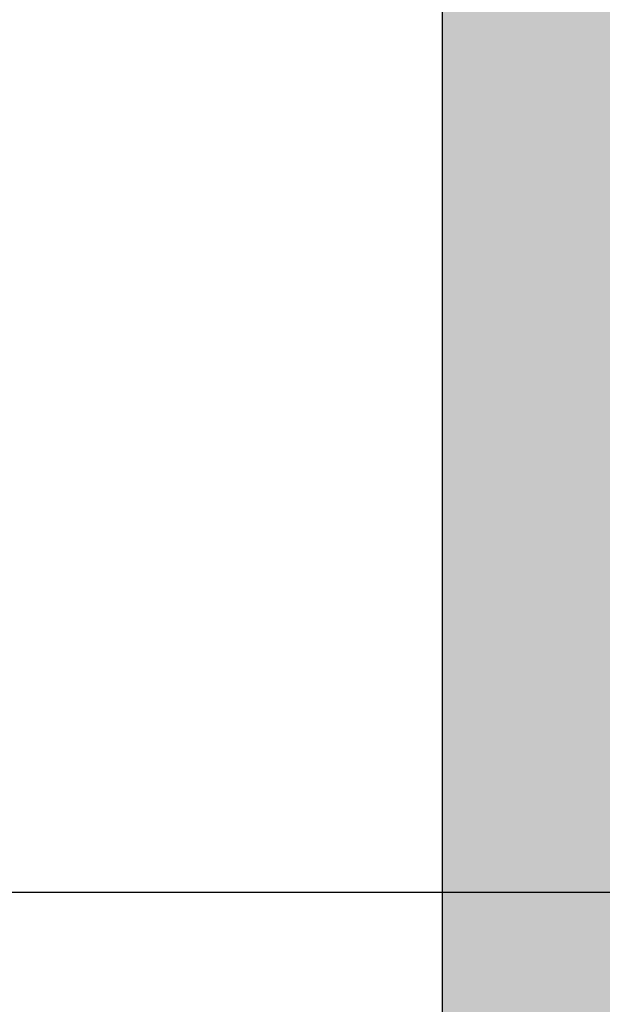
# Model space of a CAD drawing. Units: millimetres. Extents: x -22994 to 29398, y -19990 to 20176.
# Tile 37 of 135: x 190.48 to 197.67, y 29.61 to 41.76. Entities that reach past the tile are written whole.
import ezdxf
from ezdxf import colors
from ezdxf.entities.mleader import LeaderData, LeaderLine
from ezdxf.math import Vec2, Vec3

# ---------------------------------------------------------------- set-up
doc = ezdxf.new("R2010")
doc.units = ezdxf.units.MM
doc.header["$MEASUREMENT"] = 0
for name, color, linetype, lineweight in [('M-ANNO-TEXT', 7, 'Continuous', 25), ('M-DIMS', 2, 'Continuous', 18), ('M-EQPM', 7, 'Continuous', 25), ('M-EQPM-PATT', 7, 'Continuous', 18)]:
    doc.layers.add(name, color=color, linetype=linetype, lineweight=lineweight)
doc.styles.get("Standard").update_dxf_attribs({"font": 'arial.ttf'})
doc.dimstyles.get("Standard").update_dxf_attribs({"dimtxt": 0.18, "dimasz": 10000, "dimexe": 0.18, "dimexo": 0.0625, "dimgap": 0.09, "dimtad": 0, "dimtih": 1, "dimtoh": 1, "dimdec": 0, "dimzin": 0, "dimdsep": 46, "dimtxsty": 'Standard', "dimcen": 0.09, "dimadec": 0, "dimazin": 0, "dimtfac": 1, "dimtdec": 0, "dimtofl": 0, "dimtmove": 0, "dimatfit": 3, "dimfxl": 1, "dimtolj": 1, "dimtzin": 0, "dimlwd": 30, "dimarcsym": 0})

# ---------------------------------------------------------------- blocks, each defined once
blk = doc.blocks.new('*D2')
at = {"layer": 'Defpoints', "color": 0, "transparency": 16777216}
for p in [(6.677, 10.271), (290.852, 10.271), (290.852, -5.079)]:
    blk.add_point(p, dxfattribs=at)
at = {"layer": 'M-DIMS', "color": 0, "lineweight": -2, "transparency": 16777216}
for p, q in [((6.677, 10.209), (6.677, -5.259)), ((290.852, 10.209), (290.852, -5.259))]:
    blk.add_line(p, q, dxfattribs=at)
at = {"layer": 'M-DIMS', "color": 0, "lineweight": 30, "transparency": 16777216}
for p, q in [((-9993.323, -5.079), (-19993.323, -5.079)), ((10290.852, -5.079), (20290.852, -5.079))]:
    blk.add_line(p, q, dxfattribs=at)
at = {"layer": 'M-DIMS', "color": 0, "transparency": 16777216}
for points in [[(-9993.323, 1661.588), (-9993.323, -1671.745), (6.677, -5.079)], [(10290.852, 1661.588), (10290.852, -1671.745), (290.852, -5.079)]]:
    blk.add_solid(points, dxfattribs=at)
at = {"layer": 'M-DIMS', "color": 0, "transparency": 16777216, "insert": (148.765, -5.079), "char_height": 0.18, "attachment_point": 5}
blk.add_mtext('\\A1;284.2', dxfattribs=at)
blk = doc.blocks.new('*D3')
at = {"layer": 'Defpoints', "color": 0, "transparency": 16777216}
for p in [(110.265, 204.165), (110.265, 176.366), (95.833, 127.967)]:
    blk.add_point(p, dxfattribs=at)
at = {"layer": 'M-DIMS', "color": 0, "lineweight": -2, "transparency": 16777216}
for p, q in [((95.833, 128.03), (95.833, 204.345)), ((110.265, 176.429), (110.265, 204.345))]:
    blk.add_line(p, q, dxfattribs=at)
at = {"layer": 'M-DIMS', "color": 0, "lineweight": 30, "transparency": 16777216}
for p, q in [((-9904.167, 204.165), (-19904.167, 204.165)), ((10110.265, 204.165), (20110.265, 204.165))]:
    blk.add_line(p, q, dxfattribs=at)
at = {"layer": 'M-DIMS', "color": 0, "transparency": 16777216}
for points in [[(-9904.167, 1870.832), (-9904.167, -1462.501), (95.833, 204.165)], [(10110.265, 1870.832), (10110.265, -1462.501), (110.265, 204.165)]]:
    blk.add_solid(points, dxfattribs=at)
at = {"layer": 'M-DIMS', "color": 0, "transparency": 16777216, "insert": (103.049, 204.165), "char_height": 0.18, "attachment_point": 5}
blk.add_mtext('\\A1;14.432', dxfattribs=at)
blk = doc.blocks.new('*D4')
at = {"layer": 'Defpoints', "color": 0, "transparency": 16777216}
for p in [(116.265, 204.165), (110.265, 176.366), (116.265, 176.366)]:
    blk.add_point(p, dxfattribs=at)
at = {"layer": 'M-DIMS', "color": 0, "lineweight": -2, "transparency": 16777216}
for p, q in [((110.265, 176.429), (110.265, 204.345)), ((116.265, 176.429), (116.265, 204.345))]:
    blk.add_line(p, q, dxfattribs=at)
at = {"layer": 'M-DIMS', "color": 0, "lineweight": 30, "transparency": 16777216}
for p, q in [((-9889.735, 204.165), (-19889.735, 204.165)), ((10116.265, 204.165), (20116.265, 204.165))]:
    blk.add_line(p, q, dxfattribs=at)
at = {"layer": 'M-DIMS', "color": 0, "transparency": 16777216}
for points in [[(-9889.735, 1870.832), (-9889.735, -1462.501), (110.265, 204.165)], [(10116.265, 1870.832), (10116.265, -1462.501), (116.265, 204.165)]]:
    blk.add_solid(points, dxfattribs=at)
at = {"layer": 'M-DIMS', "color": 0, "transparency": 16777216, "insert": (113.265, 204.165), "char_height": 0.18, "attachment_point": 5}
blk.add_mtext('\\A1;6', dxfattribs=at)
blk = doc.blocks.new('*D5')
at = {"layer": 'Defpoints', "color": 0, "transparency": 16777216}
for p in [(181.265, 204.165), (116.265, 176.366), (181.265, 176.366)]:
    blk.add_point(p, dxfattribs=at)
at = {"layer": 'M-DIMS', "color": 0, "lineweight": -2, "transparency": 16777216}
for p, q in [((116.265, 176.429), (116.265, 204.345)), ((181.265, 176.429), (181.265, 204.345))]:
    blk.add_line(p, q, dxfattribs=at)
at = {"layer": 'M-DIMS', "color": 0, "lineweight": 30, "transparency": 16777216}
for p, q in [((-9883.735, 204.165), (-19883.735, 204.165)), ((10181.265, 204.165), (20181.265, 204.165))]:
    blk.add_line(p, q, dxfattribs=at)
at = {"layer": 'M-DIMS', "color": 0, "transparency": 16777216}
for points in [[(-9883.735, 1870.832), (-9883.735, -1462.501), (116.265, 204.165)], [(10181.265, 1870.832), (10181.265, -1462.501), (181.265, 204.165)]]:
    blk.add_solid(points, dxfattribs=at)
at = {"layer": 'M-DIMS', "color": 0, "transparency": 16777216, "insert": (148.765, 204.165), "char_height": 0.18, "attachment_point": 5}
blk.add_mtext('\\A1;65', dxfattribs=at)
blk = doc.blocks.new('*D6')
at = {"layer": 'Defpoints', "color": 0, "transparency": 16777216}
for p in [(187.265, 204.165), (181.265, 176.366), (187.265, 176.366)]:
    blk.add_point(p, dxfattribs=at)
at = {"layer": 'M-DIMS', "color": 0, "lineweight": -2, "transparency": 16777216}
for p, q in [((181.265, 176.429), (181.265, 204.345)), ((187.265, 176.429), (187.265, 204.345))]:
    blk.add_line(p, q, dxfattribs=at)
at = {"layer": 'M-DIMS', "color": 0, "lineweight": 30, "transparency": 16777216}
for p, q in [((-9818.735, 204.165), (-19818.735, 204.165)), ((10187.265, 204.165), (20187.265, 204.165))]:
    blk.add_line(p, q, dxfattribs=at)
at = {"layer": 'M-DIMS', "color": 0, "transparency": 16777216}
for points in [[(-9818.735, 1870.832), (-9818.735, -1462.501), (181.265, 204.165)], [(10187.265, 1870.832), (10187.265, -1462.501), (187.265, 204.165)]]:
    blk.add_solid(points, dxfattribs=at)
at = {"layer": 'M-DIMS', "color": 0, "transparency": 16777216, "insert": (184.265, 204.165), "char_height": 0.18, "attachment_point": 5}
blk.add_mtext('\\A1;6', dxfattribs=at)
blk = doc.blocks.new('*D7')
at = {"layer": 'Defpoints', "color": 0, "transparency": 16777216}
for p in [(201.697, 204.165), (187.265, 176.366), (201.697, 127.967)]:
    blk.add_point(p, dxfattribs=at)
at = {"layer": 'M-DIMS', "color": 0, "lineweight": -2, "transparency": 16777216}
for p, q in [((187.265, 176.429), (187.265, 204.345)), ((201.697, 128.03), (201.697, 204.345))]:
    blk.add_line(p, q, dxfattribs=at)
at = {"layer": 'M-DIMS', "color": 0, "lineweight": 30, "transparency": 16777216}
for p, q in [((-9812.735, 204.165), (-19812.735, 204.165)), ((10201.697, 204.165), (20201.697, 204.165))]:
    blk.add_line(p, q, dxfattribs=at)
at = {"layer": 'M-DIMS', "color": 0, "transparency": 16777216}
for points in [[(-9812.735, 1870.832), (-9812.735, -1462.501), (187.265, 204.165)], [(10201.697, 1870.832), (10201.697, -1462.501), (201.697, 204.165)]]:
    blk.add_solid(points, dxfattribs=at)
at = {"layer": 'M-DIMS', "color": 0, "transparency": 16777216, "insert": (194.481, 204.165), "char_height": 0.18, "attachment_point": 5}
blk.add_mtext('\\A1;14.432', dxfattribs=at)
blk = doc.blocks.new('*D8')
at = {"layer": 'Defpoints', "color": 0, "transparency": 16777216}
for p in [(227.648, 204.165), (227.648, 146.73), (201.697, 127.967)]:
    blk.add_point(p, dxfattribs=at)
at = {"layer": 'M-DIMS', "color": 0, "lineweight": -2, "transparency": 16777216}
for p, q in [((201.697, 128.03), (201.697, 204.345)), ((227.648, 146.792), (227.648, 204.345))]:
    blk.add_line(p, q, dxfattribs=at)
at = {"layer": 'M-DIMS', "color": 0, "lineweight": 30, "transparency": 16777216}
for p, q in [((-9798.303, 204.165), (-19798.303, 204.165)), ((10227.648, 204.165), (20227.648, 204.165))]:
    blk.add_line(p, q, dxfattribs=at)
at = {"layer": 'M-DIMS', "color": 0, "transparency": 16777216}
for points in [[(-9798.303, 1870.832), (-9798.303, -1462.501), (201.697, 204.165)], [(10227.648, 1870.832), (10227.648, -1462.501), (227.648, 204.165)]]:
    blk.add_solid(points, dxfattribs=at)
at = {"layer": 'M-DIMS', "color": 0, "transparency": 16777216, "insert": (214.673, 204.165), "char_height": 0.18, "attachment_point": 5}
blk.add_mtext('\\A1;25.95', dxfattribs=at)
blk = doc.blocks.new('*D9')
at = {"layer": 'Defpoints', "color": 0, "transparency": 16777216}
for p in [(187.265, 176.366), (306.202, 176.366), (290.852, 10.271)]:
    blk.add_point(p, dxfattribs=at)
at = {"layer": 'M-DIMS', "color": 0, "lineweight": 30, "transparency": 16777216}
for p, q in [((306.202, 10176.366), (306.202, 20176.366)), ((306.202, -9989.729), (306.202, -19989.729))]:
    blk.add_line(p, q, dxfattribs=at)
at = {"layer": 'M-DIMS', "color": 0, "lineweight": -2, "transparency": 16777216}
for p, q in [((187.327, 176.366), (306.382, 176.366)), ((290.915, 10.271), (306.382, 10.271))]:
    blk.add_line(p, q, dxfattribs=at)
at = {"layer": 'M-DIMS', "color": 0, "transparency": 16777216}
for points in [[(-1360.465, 10176.366), (1972.869, 10176.366), (306.202, 176.366)], [(-1360.465, -9989.729), (1972.869, -9989.729), (306.202, 10.271)]]:
    blk.add_solid(points, dxfattribs=at)
at = {"layer": 'M-DIMS', "color": 0, "transparency": 16777216, "insert": (306.202, 93.319), "char_height": 0.18, "attachment_point": 5}
blk.add_mtext('\\A1;166.1', dxfattribs=at)
blk = doc.blocks.new('*D10')
at = {"layer": 'Defpoints', "color": 0, "transparency": 16777216}
for p in [(125.65, 136.071), (133.346, 136.071), (133.346, -5.079)]:
    blk.add_point(p, dxfattribs=at)
at = {"layer": 'M-DIMS', "color": 0, "lineweight": -2, "transparency": 16777216}
for p, q in [((125.65, 136.009), (125.65, -5.259)), ((133.346, 136.009), (133.346, -5.259))]:
    blk.add_line(p, q, dxfattribs=at)
at = {"layer": 'M-DIMS', "color": 0, "lineweight": 30, "transparency": 16777216}
for p, q in [((-9874.35, -5.079), (-19874.35, -5.079)), ((10133.346, -5.079), (20133.346, -5.079))]:
    blk.add_line(p, q, dxfattribs=at)
at = {"layer": 'M-DIMS', "color": 0, "transparency": 16777216}
for points in [[(-9874.35, 1661.588), (-9874.35, -1671.745), (125.65, -5.079)], [(10133.346, 1661.588), (10133.346, -1671.745), (133.346, -5.079)]]:
    blk.add_solid(points, dxfattribs=at)
at = {"layer": 'M-DIMS', "color": 0, "transparency": 16777216, "insert": (129.498, -5.079), "char_height": 0.18, "attachment_point": 5}
blk.add_mtext('\\A1;7.696', dxfattribs=at)
blk = doc.blocks.new('*D11')
at = {"layer": 'Defpoints', "color": 0, "transparency": 16777216}
for p in [(133.346, 136.071), (135.65, 136.071), (135.65, -5.079)]:
    blk.add_point(p, dxfattribs=at)
at = {"layer": 'M-DIMS', "color": 0, "lineweight": -2, "transparency": 16777216}
for p, q in [((133.346, 136.009), (133.346, -5.259)), ((135.65, 136.009), (135.65, -5.259))]:
    blk.add_line(p, q, dxfattribs=at)
at = {"layer": 'M-DIMS', "color": 0, "lineweight": 30, "transparency": 16777216}
for p, q in [((-9866.654, -5.079), (-19866.654, -5.079)), ((10135.65, -5.079), (20135.65, -5.079))]:
    blk.add_line(p, q, dxfattribs=at)
at = {"layer": 'M-DIMS', "color": 0, "transparency": 16777216}
for points in [[(-9866.654, 1661.588), (-9866.654, -1671.745), (133.346, -5.079)], [(10135.65, 1661.588), (10135.65, -1671.745), (135.65, -5.079)]]:
    blk.add_solid(points, dxfattribs=at)
at = {"layer": 'M-DIMS', "color": 0, "transparency": 16777216, "insert": (134.498, -5.079), "char_height": 0.18, "attachment_point": 5}
blk.add_mtext('\\A1;2.304', dxfattribs=at)
blk = doc.blocks.new('*D12')
at = {"layer": 'Defpoints', "color": 0, "transparency": 16777216}
for p in [(135.65, 136.071), (145.65, 136.071), (145.65, -5.079)]:
    blk.add_point(p, dxfattribs=at)
at = {"layer": 'M-DIMS', "color": 0, "lineweight": -2, "transparency": 16777216}
for p, q in [((135.65, 136.009), (135.65, -5.259)), ((145.65, 136.009), (145.65, -5.259))]:
    blk.add_line(p, q, dxfattribs=at)
at = {"layer": 'M-DIMS', "color": 0, "lineweight": 30, "transparency": 16777216}
for p, q in [((-9864.35, -5.079), (-19864.35, -5.079)), ((10145.65, -5.079), (20145.65, -5.079))]:
    blk.add_line(p, q, dxfattribs=at)
at = {"layer": 'M-DIMS', "color": 0, "transparency": 16777216}
for points in [[(-9864.35, 1661.588), (-9864.35, -1671.745), (135.65, -5.079)], [(10145.65, 1661.588), (10145.65, -1671.745), (145.65, -5.079)]]:
    blk.add_solid(points, dxfattribs=at)
at = {"layer": 'M-DIMS', "color": 0, "transparency": 16777216, "insert": (140.65, -5.079), "char_height": 0.18, "attachment_point": 5}
blk.add_mtext('\\A1;10', dxfattribs=at)
blk = doc.blocks.new('*D13')
at = {"layer": 'Defpoints', "color": 0, "transparency": 16777216}
for p in [(145.65, 136.071), (155.65, 136.071), (155.65, -5.079)]:
    blk.add_point(p, dxfattribs=at)
at = {"layer": 'M-DIMS', "color": 0, "lineweight": -2, "transparency": 16777216}
for p, q in [((145.65, 136.009), (145.65, -5.259)), ((155.65, 136.009), (155.65, -5.259))]:
    blk.add_line(p, q, dxfattribs=at)
at = {"layer": 'M-DIMS', "color": 0, "lineweight": 30, "transparency": 16777216}
for p, q in [((-9854.35, -5.079), (-19854.35, -5.079)), ((10155.65, -5.079), (20155.65, -5.079))]:
    blk.add_line(p, q, dxfattribs=at)
at = {"layer": 'M-DIMS', "color": 0, "transparency": 16777216}
for points in [[(-9854.35, 1661.588), (-9854.35, -1671.745), (145.65, -5.079)], [(10155.65, 1661.588), (10155.65, -1671.745), (155.65, -5.079)]]:
    blk.add_solid(points, dxfattribs=at)
at = {"layer": 'M-DIMS', "color": 0, "transparency": 16777216, "insert": (150.65, -5.079), "char_height": 0.18, "attachment_point": 5}
blk.add_mtext('\\A1;10', dxfattribs=at)
blk = doc.blocks.new('*D14')
at = {"layer": 'Defpoints', "color": 0, "transparency": 16777216}
for p in [(155.65, 136.071), (165.65, 136.071), (165.65, -5.079)]:
    blk.add_point(p, dxfattribs=at)
at = {"layer": 'M-DIMS', "color": 0, "lineweight": -2, "transparency": 16777216}
for p, q in [((155.65, 136.009), (155.65, -5.259)), ((165.65, 136.009), (165.65, -5.259))]:
    blk.add_line(p, q, dxfattribs=at)
at = {"layer": 'M-DIMS', "color": 0, "lineweight": 30, "transparency": 16777216}
for p, q in [((-9844.35, -5.079), (-19844.35, -5.079)), ((10165.65, -5.079), (20165.65, -5.079))]:
    blk.add_line(p, q, dxfattribs=at)
at = {"layer": 'M-DIMS', "color": 0, "transparency": 16777216}
for points in [[(-9844.35, 1661.588), (-9844.35, -1671.745), (155.65, -5.079)], [(10165.65, 1661.588), (10165.65, -1671.745), (165.65, -5.079)]]:
    blk.add_solid(points, dxfattribs=at)
at = {"layer": 'M-DIMS', "color": 0, "transparency": 16777216, "insert": (160.65, -5.079), "char_height": 0.18, "attachment_point": 5}
blk.add_mtext('\\A1;10', dxfattribs=at)
blk = doc.blocks.new('*D15')
at = {"layer": 'Defpoints', "color": 0, "transparency": 16777216}
for p in [(173.346, 154.788), (173.346, 136.071), (306.202, 136.071)]:
    blk.add_point(p, dxfattribs=at)
at = {"layer": 'M-DIMS', "color": 0, "lineweight": 30, "transparency": 16777216}
for p, q in [((306.202, 10154.788), (306.202, 20154.788)), ((306.202, -9863.929), (306.202, -19863.929))]:
    blk.add_line(p, q, dxfattribs=at)
at = {"layer": 'M-DIMS', "color": 0, "lineweight": -2, "transparency": 16777216}
for p, q in [((173.408, 154.788), (306.382, 154.788)), ((173.408, 136.071), (306.382, 136.071))]:
    blk.add_line(p, q, dxfattribs=at)
at = {"layer": 'M-DIMS', "color": 0, "transparency": 16777216}
for points in [[(-1360.465, 10154.788), (1972.869, 10154.788), (306.202, 154.788)], [(-1360.465, -9863.929), (1972.869, -9863.929), (306.202, 136.071)]]:
    blk.add_solid(points, dxfattribs=at)
at = {"layer": 'M-DIMS', "color": 0, "transparency": 16777216, "insert": (306.202, 145.43), "char_height": 0.18, "attachment_point": 5}
blk.add_mtext('\\A1;18.717', dxfattribs=at)
blk = doc.blocks.new('*D16')
at = {"layer": 'Defpoints', "color": 0, "transparency": 16777216}
for p in [(120.17, 204.165), (110.466, 48.035), (120.17, 48.035)]:
    blk.add_point(p, dxfattribs=at)
at = {"layer": 'M-DIMS', "color": 0, "lineweight": -2, "transparency": 16777216}
for p, q in [((110.466, 48.097), (110.466, 204.345)), ((120.17, 48.097), (120.17, 204.345))]:
    blk.add_line(p, q, dxfattribs=at)
at = {"layer": 'M-DIMS', "color": 0, "lineweight": 30, "transparency": 16777216}
for p, q in [((-9889.534, 204.165), (-19889.534, 204.165)), ((10120.17, 204.165), (20120.17, 204.165))]:
    blk.add_line(p, q, dxfattribs=at)
at = {"layer": 'M-DIMS', "color": 0, "transparency": 16777216}
for points in [[(-9889.534, 1870.832), (-9889.534, -1462.501), (110.466, 204.165)], [(10120.17, 1870.832), (10120.17, -1462.501), (120.17, 204.165)]]:
    blk.add_solid(points, dxfattribs=at)
at = {"layer": 'M-DIMS', "color": 0, "transparency": 16777216, "insert": (115.318, 204.165), "char_height": 0.18, "attachment_point": 5}
blk.add_mtext('\\A1;9.704', dxfattribs=at)
blk = doc.blocks.new('*D17')
at = {"layer": 'Defpoints', "color": 0, "transparency": 16777216}
for p in [(126.17, 204.165), (120.17, 48.035), (126.17, 48.035)]:
    blk.add_point(p, dxfattribs=at)
at = {"layer": 'M-DIMS', "color": 0, "lineweight": -2, "transparency": 16777216}
for p, q in [((120.17, 48.097), (120.17, 204.345)), ((126.17, 48.097), (126.17, 204.345))]:
    blk.add_line(p, q, dxfattribs=at)
at = {"layer": 'M-DIMS', "color": 0, "lineweight": 30, "transparency": 16777216}
for p, q in [((-9879.83, 204.165), (-19879.83, 204.165)), ((10126.17, 204.165), (20126.17, 204.165))]:
    blk.add_line(p, q, dxfattribs=at)
at = {"layer": 'M-DIMS', "color": 0, "transparency": 16777216}
for points in [[(-9879.83, 1870.832), (-9879.83, -1462.501), (120.17, 204.165)], [(10126.17, 1870.832), (10126.17, -1462.501), (126.17, 204.165)]]:
    blk.add_solid(points, dxfattribs=at)
at = {"layer": 'M-DIMS', "color": 0, "transparency": 16777216, "insert": (123.17, 204.165), "char_height": 0.18, "attachment_point": 5}
blk.add_mtext('\\A1;6', dxfattribs=at)
blk = doc.blocks.new('*D18')
at = {"layer": 'Defpoints', "color": 0, "transparency": 16777216}
for p in [(132.17, 204.165), (126.17, 48.035), (132.17, 48.035)]:
    blk.add_point(p, dxfattribs=at)
at = {"layer": 'M-DIMS', "color": 0, "lineweight": -2, "transparency": 16777216}
for p, q in [((126.17, 48.097), (126.17, 204.345)), ((132.17, 48.097), (132.17, 204.345))]:
    blk.add_line(p, q, dxfattribs=at)
at = {"layer": 'M-DIMS', "color": 0, "lineweight": 30, "transparency": 16777216}
for p, q in [((-9873.83, 204.165), (-19873.83, 204.165)), ((10132.17, 204.165), (20132.17, 204.165))]:
    blk.add_line(p, q, dxfattribs=at)
at = {"layer": 'M-DIMS', "color": 0, "transparency": 16777216}
for points in [[(-9873.83, 1870.832), (-9873.83, -1462.501), (126.17, 204.165)], [(10132.17, 1870.832), (10132.17, -1462.501), (132.17, 204.165)]]:
    blk.add_solid(points, dxfattribs=at)
at = {"layer": 'M-DIMS', "color": 0, "transparency": 16777216, "insert": (129.17, 204.165), "char_height": 0.18, "attachment_point": 5}
blk.add_mtext('\\A1;6', dxfattribs=at)
blk = doc.blocks.new('*D19')
at = {"layer": 'Defpoints', "color": 0, "transparency": 16777216}
for p in [(138.17, 204.165), (132.17, 48.035), (138.17, 48.035)]:
    blk.add_point(p, dxfattribs=at)
at = {"layer": 'M-DIMS', "color": 0, "lineweight": -2, "transparency": 16777216}
for p, q in [((132.17, 48.097), (132.17, 204.345)), ((138.17, 48.097), (138.17, 204.345))]:
    blk.add_line(p, q, dxfattribs=at)
at = {"layer": 'M-DIMS', "color": 0, "lineweight": 30, "transparency": 16777216}
for p, q in [((-9867.83, 204.165), (-19867.83, 204.165)), ((10138.17, 204.165), (20138.17, 204.165))]:
    blk.add_line(p, q, dxfattribs=at)
at = {"layer": 'M-DIMS', "color": 0, "transparency": 16777216}
for points in [[(-9867.83, 1870.832), (-9867.83, -1462.501), (132.17, 204.165)], [(10138.17, 1870.832), (10138.17, -1462.501), (138.17, 204.165)]]:
    blk.add_solid(points, dxfattribs=at)
at = {"layer": 'M-DIMS', "color": 0, "transparency": 16777216, "insert": (135.17, 204.165), "char_height": 0.18, "attachment_point": 5}
blk.add_mtext('\\A1;6', dxfattribs=at)
blk = doc.blocks.new('*D20')
at = {"layer": 'Defpoints', "color": 0, "transparency": 16777216}
for p in [(144.17, 204.165), (138.17, 48.035), (144.17, 48.035)]:
    blk.add_point(p, dxfattribs=at)
at = {"layer": 'M-DIMS', "color": 0, "lineweight": -2, "transparency": 16777216}
for p, q in [((138.17, 48.097), (138.17, 204.345)), ((144.17, 48.097), (144.17, 204.345))]:
    blk.add_line(p, q, dxfattribs=at)
at = {"layer": 'M-DIMS', "color": 0, "lineweight": 30, "transparency": 16777216}
for p, q in [((-9861.83, 204.165), (-19861.83, 204.165)), ((10144.17, 204.165), (20144.17, 204.165))]:
    blk.add_line(p, q, dxfattribs=at)
at = {"layer": 'M-DIMS', "color": 0, "transparency": 16777216}
for points in [[(-9861.83, 1870.832), (-9861.83, -1462.501), (138.17, 204.165)], [(10144.17, 1870.832), (10144.17, -1462.501), (144.17, 204.165)]]:
    blk.add_solid(points, dxfattribs=at)
at = {"layer": 'M-DIMS', "color": 0, "transparency": 16777216, "insert": (141.17, 204.165), "char_height": 0.18, "attachment_point": 5}
blk.add_mtext('\\A1;6', dxfattribs=at)
blk = doc.blocks.new('*D21')
at = {"layer": 'Defpoints', "color": 0, "transparency": 16777216}
for p in [(149.116, 204.165), (144.17, 48.035), (149.116, 48.035)]:
    blk.add_point(p, dxfattribs=at)
at = {"layer": 'M-DIMS', "color": 0, "lineweight": -2, "transparency": 16777216}
for p, q in [((144.17, 48.097), (144.17, 204.345)), ((149.116, 48.097), (149.116, 204.345))]:
    blk.add_line(p, q, dxfattribs=at)
at = {"layer": 'M-DIMS', "color": 0, "lineweight": 30, "transparency": 16777216}
for p, q in [((-9855.83, 204.165), (-19855.83, 204.165)), ((10149.116, 204.165), (20149.116, 204.165))]:
    blk.add_line(p, q, dxfattribs=at)
at = {"layer": 'M-DIMS', "color": 0, "transparency": 16777216}
for points in [[(-9855.83, 1870.832), (-9855.83, -1462.501), (144.17, 204.165)], [(10149.116, 1870.832), (10149.116, -1462.501), (149.116, 204.165)]]:
    blk.add_solid(points, dxfattribs=at)
at = {"layer": 'M-DIMS', "color": 0, "transparency": 16777216, "insert": (146.643, 204.165), "char_height": 0.18, "attachment_point": 5}
blk.add_mtext('\\A1;4.945', dxfattribs=at)
blk = doc.blocks.new('*D22')
at = {"layer": 'Defpoints', "color": 0, "transparency": 16777216}
for p in [(149.116, 30.99), (155.116, 30.99), (155.116, -5.079)]:
    blk.add_point(p, dxfattribs=at)
at = {"layer": 'M-DIMS', "color": 0, "lineweight": -2, "transparency": 16777216}
for p, q in [((149.116, 30.927), (149.116, -5.259)), ((155.116, 30.927), (155.116, -5.259))]:
    blk.add_line(p, q, dxfattribs=at)
at = {"layer": 'M-DIMS', "color": 0, "lineweight": 30, "transparency": 16777216}
for p, q in [((-9850.884, -5.079), (-19850.884, -5.079)), ((10155.116, -5.079), (20155.116, -5.079))]:
    blk.add_line(p, q, dxfattribs=at)
at = {"layer": 'M-DIMS', "color": 0, "transparency": 16777216}
for points in [[(-9850.884, 1661.588), (-9850.884, -1671.745), (149.116, -5.079)], [(10155.116, 1661.588), (10155.116, -1671.745), (155.116, -5.079)]]:
    blk.add_solid(points, dxfattribs=at)
at = {"layer": 'M-DIMS', "color": 0, "transparency": 16777216, "insert": (152.116, -5.079), "char_height": 0.18, "attachment_point": 5}
blk.add_mtext('\\A1;6', dxfattribs=at)
blk = doc.blocks.new('*D23')
at = {"layer": 'Defpoints', "color": 0, "transparency": 16777216}
for p in [(155.116, 30.99), (161.116, 30.99), (161.116, -5.079)]:
    blk.add_point(p, dxfattribs=at)
at = {"layer": 'M-DIMS', "color": 0, "lineweight": -2, "transparency": 16777216}
for p, q in [((155.116, 30.927), (155.116, -5.259)), ((161.116, 30.927), (161.116, -5.259))]:
    blk.add_line(p, q, dxfattribs=at)
at = {"layer": 'M-DIMS', "color": 0, "lineweight": 30, "transparency": 16777216}
for p, q in [((-9844.884, -5.079), (-19844.884, -5.079)), ((10161.116, -5.079), (20161.116, -5.079))]:
    blk.add_line(p, q, dxfattribs=at)
at = {"layer": 'M-DIMS', "color": 0, "transparency": 16777216}
for points in [[(-9844.884, 1661.588), (-9844.884, -1671.745), (155.116, -5.079)], [(10161.116, 1661.588), (10161.116, -1671.745), (161.116, -5.079)]]:
    blk.add_solid(points, dxfattribs=at)
at = {"layer": 'M-DIMS', "color": 0, "transparency": 16777216, "insert": (158.116, -5.079), "char_height": 0.18, "attachment_point": 5}
blk.add_mtext('\\A1;6', dxfattribs=at)
blk = doc.blocks.new('*D24')
at = {"layer": 'Defpoints', "color": 0, "transparency": 16777216}
for p in [(161.116, 30.99), (166.439, 30.99), (166.439, -5.079)]:
    blk.add_point(p, dxfattribs=at)
at = {"layer": 'M-DIMS', "color": 0, "lineweight": -2, "transparency": 16777216}
for p, q in [((161.116, 30.927), (161.116, -5.259)), ((166.439, 30.927), (166.439, -5.259))]:
    blk.add_line(p, q, dxfattribs=at)
at = {"layer": 'M-DIMS', "color": 0, "lineweight": 30, "transparency": 16777216}
for p, q in [((-9838.884, -5.079), (-19838.884, -5.079)), ((10166.439, -5.079), (20166.439, -5.079))]:
    blk.add_line(p, q, dxfattribs=at)
at = {"layer": 'M-DIMS', "color": 0, "transparency": 16777216}
for points in [[(-9838.884, 1661.588), (-9838.884, -1671.745), (161.116, -5.079)], [(10166.439, 1661.588), (10166.439, -1671.745), (166.439, -5.079)]]:
    blk.add_solid(points, dxfattribs=at)
at = {"layer": 'M-DIMS', "color": 0, "transparency": 16777216, "insert": (163.777, -5.079), "char_height": 0.18, "attachment_point": 5}
blk.add_mtext('\\A1;5.323', dxfattribs=at)
blk = doc.blocks.new('*D25')
at = {"layer": 'Defpoints', "color": 0, "transparency": 16777216}
for p in [(166.439, 30.99), (172.439, 30.99), (172.439, -5.079)]:
    blk.add_point(p, dxfattribs=at)
at = {"layer": 'M-DIMS', "color": 0, "lineweight": -2, "transparency": 16777216}
for p, q in [((166.439, 30.927), (166.439, -5.259)), ((172.439, 30.927), (172.439, -5.259))]:
    blk.add_line(p, q, dxfattribs=at)
at = {"layer": 'M-DIMS', "color": 0, "lineweight": 30, "transparency": 16777216}
for p, q in [((-9833.561, -5.079), (-19833.561, -5.079)), ((10172.439, -5.079), (20172.439, -5.079))]:
    blk.add_line(p, q, dxfattribs=at)
at = {"layer": 'M-DIMS', "color": 0, "transparency": 16777216}
for points in [[(-9833.561, 1661.588), (-9833.561, -1671.745), (166.439, -5.079)], [(10172.439, 1661.588), (10172.439, -1671.745), (172.439, -5.079)]]:
    blk.add_solid(points, dxfattribs=at)
at = {"layer": 'M-DIMS', "color": 0, "transparency": 16777216, "insert": (169.439, -5.079), "char_height": 0.18, "attachment_point": 5}
blk.add_mtext('\\A1;6', dxfattribs=at)
blk = doc.blocks.new('*D26')
at = {"layer": 'Defpoints', "color": 0, "transparency": 16777216}
for p in [(172.439, 30.99), (178.439, 30.99), (178.439, -5.079)]:
    blk.add_point(p, dxfattribs=at)
at = {"layer": 'M-DIMS', "color": 0, "lineweight": -2, "transparency": 16777216}
for p, q in [((172.439, 30.927), (172.439, -5.259)), ((178.439, 30.927), (178.439, -5.259))]:
    blk.add_line(p, q, dxfattribs=at)
at = {"layer": 'M-DIMS', "color": 0, "lineweight": 30, "transparency": 16777216}
for p, q in [((-9827.561, -5.079), (-19827.561, -5.079)), ((10178.439, -5.079), (20178.439, -5.079))]:
    blk.add_line(p, q, dxfattribs=at)
at = {"layer": 'M-DIMS', "color": 0, "transparency": 16777216}
for points in [[(-9827.561, 1661.588), (-9827.561, -1671.745), (172.439, -5.079)], [(10178.439, 1661.588), (10178.439, -1671.745), (178.439, -5.079)]]:
    blk.add_solid(points, dxfattribs=at)
at = {"layer": 'M-DIMS', "color": 0, "transparency": 16777216, "insert": (175.439, -5.079), "char_height": 0.18, "attachment_point": 5}
blk.add_mtext('\\A1;6', dxfattribs=at)
blk = doc.blocks.new('*D27')
at = {"layer": 'Defpoints', "color": 0, "transparency": 16777216}
for p in [(178.439, 30.99), (188.117, 30.99), (188.117, -5.079)]:
    blk.add_point(p, dxfattribs=at)
at = {"layer": 'M-DIMS', "color": 0, "lineweight": -2, "transparency": 16777216}
for p, q in [((178.439, 30.927), (178.439, -5.259)), ((188.117, 30.927), (188.117, -5.259))]:
    blk.add_line(p, q, dxfattribs=at)
at = {"layer": 'M-DIMS', "color": 0, "lineweight": 30, "transparency": 16777216}
for p, q in [((-9821.561, -5.079), (-19821.561, -5.079)), ((10188.117, -5.079), (20188.117, -5.079))]:
    blk.add_line(p, q, dxfattribs=at)
at = {"layer": 'M-DIMS', "color": 0, "transparency": 16777216}
for points in [[(-9821.561, 1661.588), (-9821.561, -1671.745), (178.439, -5.079)], [(10188.117, 1661.588), (10188.117, -1671.745), (188.117, -5.079)]]:
    blk.add_solid(points, dxfattribs=at)
at = {"layer": 'M-DIMS', "color": 0, "transparency": 16777216, "insert": (183.278, -5.079), "char_height": 0.18, "attachment_point": 5}
blk.add_mtext('\\A1;9.679', dxfattribs=at)
blk = doc.blocks.new('*D28')
at = {"layer": 'Defpoints', "color": 0, "transparency": 16777216}
for p in [(188.117, 48.035), (306.202, 48.035), (188.117, 30.99)]:
    blk.add_point(p, dxfattribs=at)
at = {"layer": 'M-DIMS', "color": 0, "lineweight": 30, "transparency": 16777216}
for p, q in [((306.202, 10048.035), (306.202, 20048.035)), ((306.202, -9969.01), (306.202, -19969.01))]:
    blk.add_line(p, q, dxfattribs=at)
at = {"layer": 'M-DIMS', "color": 0, "lineweight": -2, "transparency": 16777216}
for p, q in [((188.18, 48.035), (306.382, 48.035)), ((188.18, 30.99), (306.382, 30.99))]:
    blk.add_line(p, q, dxfattribs=at)
at = {"layer": 'M-DIMS', "color": 0, "transparency": 16777216}
for points in [[(-1360.465, 10048.035), (1972.869, 10048.035), (306.202, 48.035)], [(-1360.465, -9969.01), (1972.869, -9969.01), (306.202, 30.99)]]:
    blk.add_solid(points, dxfattribs=at)
at = {"layer": 'M-DIMS', "color": 0, "transparency": 16777216, "insert": (306.202, 39.512), "char_height": 0.18, "attachment_point": 5}
blk.add_mtext('\\A1;17.045', dxfattribs=at)
blk = doc.blocks.new('*D29')
at = {"layer": 'Defpoints', "color": 0, "transparency": 16777216}
for p in [(36.801, 80.045), (64.03, 80.045)]:
    blk.add_point(p, dxfattribs=at)
at = {"layer": 'M-DIMS', "color": 0, "lineweight": -2, "transparency": 16777216}
for p, q in [((50.415, 79.955), (50.415, 80.135)), ((50.325, 80.045), (50.505, 80.045))]:
    blk.add_line(p, q, dxfattribs=at)
at = {"layer": 'M-DIMS', "color": 0, "lineweight": 30, "transparency": 16777216}
blk.add_line((20064.03, 80.03), (10064.03, 80.038), dxfattribs=at)
at = {"layer": 'M-DIMS', "color": 0, "transparency": 16777216}
blk.add_solid([(10064.031, 1746.704), (10064.028, -1586.629), (64.03, 80.045)], dxfattribs=at)
at = {"layer": 'M-DIMS', "color": 0, "transparency": 16777216, "insert": (20064.521, 80.03), "char_height": 0.18, "attachment_point": 5}
blk.add_mtext('\\A1;∅27.23', dxfattribs=at)
blk = doc.blocks.new('*D36')
at = {"layer": 'Defpoints', "color": 0, "transparency": 16777216}
for p in [(46.39, 31.303), (46.387, 26.593)]:
    blk.add_point(p, dxfattribs=at)
at = {"layer": 'M-DIMS', "color": 0, "lineweight": 30, "transparency": 16777216}
for p, q in [((57.15, 20031.301), (51.77, 10031.302)), ((10057.15, 20031.301), (57.15, 20031.301))]:
    blk.add_line(p, q, dxfattribs=at)
at = {"layer": 'M-DIMS', "color": 0, "lineweight": -2, "transparency": 16777216}
for p, q in [((46.389, 28.858), (46.389, 29.038)), ((46.299, 28.948), (46.479, 28.948))]:
    blk.add_line(p, q, dxfattribs=at)
at = {"layer": 'M-DIMS', "color": 0, "transparency": 16777216}
blk.add_solid([(-1614.896, 10032.199), (1718.436, 10030.405), (46.39, 31.303)], dxfattribs=at)
at = {"layer": 'M-DIMS', "color": 0, "transparency": 16777216, "insert": (10057.554, 20031.301), "char_height": 0.18, "attachment_point": 5}
blk.add_mtext('\\A1;∅4.71', dxfattribs=at)
blk = doc.blocks.new('*D37')
at = {"layer": 'Defpoints', "color": 0, "transparency": 16777216}
for p in [(54.834, 118.615), (59.494, 118.614)]:
    blk.add_point(p, dxfattribs=at)
at = {"layer": 'M-DIMS', "color": 0, "lineweight": -2, "transparency": 16777216}
for p, q in [((57.164, 118.524), (57.164, 118.704)), ((57.074, 118.614), (57.254, 118.614))]:
    blk.add_line(p, q, dxfattribs=at)
at = {"layer": 'M-DIMS', "color": 0, "lineweight": 30, "transparency": 16777216}
blk.add_line((20059.493, 116.253), (10059.494, 117.434), dxfattribs=at)
at = {"layer": 'M-DIMS', "color": 0, "transparency": 16777216}
blk.add_solid([(10059.69, 1784.1), (10059.297, -1549.233), (59.494, 118.614)], dxfattribs=at)
at = {"layer": 'M-DIMS', "color": 0, "transparency": 16777216, "insert": (20059.985, 116.253), "char_height": 0.18, "attachment_point": 5}
blk.add_mtext('\\A1;∅4.659', dxfattribs=at)

msp = doc.modelspace()

# ---------------------------------------------------------------- hatches: boundary and pattern name
at = {"layer": 'M-EQPM-PATT'}
h = msp.add_hatch(color=256, dxfattribs=at)
h.set_gradient(color1=(205, 32, 39), color2=(205, 32, 39), tint=1)
h.paths.add_polyline_path([(116.2647, 150.3662), (116.2647, 170.3662), (116.2647, 176.3662), (110.2647, 176.3662), (110.2647, 152.0276), (95.8327, 127.967), (95.8327, 16.6063), (201.6967, 16.6063), (201.6967, 127.967), (187.2647, 152.0276), (187.2647, 176.3662), (181.2647, 176.3662), (181.2647, 170.3662), (181.2647, 150.3662), (195.6967, 126.3055), (195.6967, 22.6063), (101.8327, 22.6063), (101.8327, 126.3055)])
h.paths.add_polyline_path([(185.2208, 88.6347), (101.8327, 88.6347), (101.8327, 87.6347), (182.8066, 87.6347), (178.7313, 83.5594), (195.6967, 83.5594), (195.6967, 84.5594), (181.1455, 84.5594)], flags=17)
h.paths.add_polyline_path([(95.8327, 88.6347), (60.9779, 88.6347, -0.0228552), (61.7178, 87.6347), (95.8327, 87.6347)])
h.paths.add_polyline_path([(215.6212, 86.5189), (215.6212, 80.5999), (220.5095, 83.5594)])
h.paths.add_polyline_path([(215.6212, 84.5594), (201.6967, 84.5594), (201.6967, 83.5594), (215.6212, 83.5594)])
h.paths.add_polyline_path([(225.3978, 86.5189), (220.5095, 83.5594), (225.3978, 80.5999)])
h.paths.add_polyline_path([(231.6256, 84.5594), (225.3978, 84.5594), (225.3978, 83.5594), (231.6256, 83.5594)])

# ---------------------------------------------------------------- linework, layer by layer
at = {"layer": 'M-EQPM'}
msp.add_lwpolyline([(116.2647, 170.3662), (116.2647, 150.3662), (101.8327, 126.3055), (101.8327, 22.6063), (195.6967, 22.6063), (195.6967, 126.3055), (181.2647, 150.3662), (181.2647, 170.3662)], dxfattribs=at)

# ---------------------------------------------------------------- dimensions: what is measured, and where the dimension line sits
at = {"layer": 'M-DIMS'}
for base, p1, p2, override, picture, middle in [((306.202, 176.3662), (290.852, 10.2713), (187.2647, 176.3662), {"dimdec": 1, "dimlfac": 1, "dimrnd": 0, "dimzin": 0, "dimdsep": 46, "dimlunit": 2}, '*D9', (306.202, 93.3187)), ((306.202, 136.0713), (173.3459, 154.788), (173.3459, 136.0713), {"dimdec": 3, "dimlfac": 1, "dimrnd": 0, "dimzin": 0, "dimdsep": 46, "dimlunit": 2}, '*D15', (306.202, 145.4297)), ((306.202, 48.0349), (188.1175, 30.9895), (188.1175, 48.0349), {"dimdec": 3, "dimlfac": 1, "dimrnd": 0, "dimzin": 0, "dimdsep": 46, "dimlunit": 2}, '*D28', (306.202, 39.5122))]:
    dim = msp.add_linear_dim(base=base, p1=p1, p2=p2, angle=90, dimstyle='Standard', override=override, dxfattribs=at)
    dim.commit()
    dim.dimension.update_dxf_attribs({"geometry": picture, "text_midpoint": middle})
dim = msp.add_diameter_dim_2p(p1=(46.3875, 26.5934), p2=(46.39, 31.3035), dimstyle='Standard', override={"dimdec": 2, "dimlfac": 1, "dimrnd": 0, "dimzin": 0, "dimdsep": 46, "dimlunit": 2}, dxfattribs=at)
dim.commit()
dim.dimension.update_dxf_attribs({"geometry": '*D36', "text_midpoint": (10057.5542, 20031.3006), "dimtype": 163})
for base, p1, p2, override, picture, middle in [((110.2647, 204.1654), (95.8327, 127.967), (110.2647, 176.3662), {"dimdec": 3, "dimlfac": 1, "dimrnd": 0, "dimzin": 0, "dimdsep": 46, "dimlunit": 2}, '*D3', (103.0487, 204.1654)), ((116.2647, 204.1654), (110.2647, 176.3662), (116.2647, 176.3662), {"dimdec": 0, "dimlfac": 1, "dimrnd": 0, "dimzin": 0, "dimdsep": 46, "dimlunit": 2}, '*D4', (113.2647, 204.1654)), ((120.1702, 204.1654), (110.4658, 48.0349), (120.1702, 48.0349), {"dimdec": 3, "dimlfac": 1, "dimrnd": 0, "dimzin": 0, "dimdsep": 46, "dimlunit": 2}, '*D16', (115.318, 204.1654)), ((181.2647, 204.1654), (116.2647, 176.3662), (181.2647, 176.3662), {"dimdec": 0, "dimlfac": 1, "dimrnd": 0, "dimzin": 0, "dimdsep": 46, "dimlunit": 2}, '*D5', (148.7647, 204.1654)), ((126.1702, 204.1654), (120.1702, 48.0349), (126.1702, 48.0349), {"dimdec": 0, "dimlfac": 1, "dimrnd": 0, "dimzin": 0, "dimdsep": 46, "dimlunit": 2}, '*D17', (123.1702, 204.1654)), ((132.1702, 204.1654), (126.1702, 48.0349), (132.1702, 48.0349), {"dimdec": 0, "dimlfac": 1, "dimrnd": 0, "dimzin": 0, "dimdsep": 46, "dimlunit": 2}, '*D18', (129.1702, 204.1654)), ((138.1702, 204.1654), (132.1702, 48.0349), (138.1702, 48.0349), {"dimdec": 0, "dimlfac": 1, "dimrnd": 0, "dimzin": 0, "dimdsep": 46, "dimlunit": 2}, '*D19', (135.1702, 204.1654)), ((144.1702, 204.1654), (138.1702, 48.0349), (144.1702, 48.0349), {"dimdec": 0, "dimlfac": 1, "dimrnd": 0, "dimzin": 0, "dimdsep": 46, "dimlunit": 2}, '*D20', (141.1702, 204.1654)), ((149.11567, 204.16539), (144.17023, 48.03494), (149.11567, 48.03494), {"dimdec": 3, "dimlfac": 1, "dimrnd": 0, "dimzin": 0, "dimdsep": 46, "dimlunit": 2}, '*D21', (146.64295, 204.16539)), ((187.2647, 204.1654), (181.2647, 176.3662), (187.2647, 176.3662), {"dimdec": 0, "dimlfac": 1, "dimrnd": 0, "dimzin": 0, "dimdsep": 46, "dimlunit": 2}, '*D6', (184.2647, 204.1654)), ((201.6967, 204.1654), (187.2647, 176.3662), (201.6967, 127.967), {"dimdec": 3, "dimlfac": 1, "dimrnd": 0, "dimzin": 0, "dimdsep": 46, "dimlunit": 2}, '*D7', (194.4807, 204.1654)), ((227.6485, 204.1654), (201.6967, 127.967), (227.6485, 146.7296), {"dimdec": 2, "dimlfac": 1, "dimrnd": 0, "dimzin": 0, "dimdsep": 46, "dimlunit": 2}, '*D8', (214.6726, 204.1654)), ((290.852, -5.0787), (6.6773, 10.2713), (290.852, 10.2713), {"dimdec": 1, "dimlfac": 1, "dimrnd": 0, "dimzin": 0, "dimdsep": 46, "dimlunit": 2}, '*D2', (148.7647, -5.0787)), ((133.3459, -5.0787), (125.6498, 136.0713), (133.3459, 136.0713), {"dimdec": 3, "dimlfac": 1, "dimrnd": 0, "dimzin": 0, "dimdsep": 46, "dimlunit": 2}, '*D10', (129.4978, -5.0787)), ((135.6498, -5.0787), (133.3459, 136.0713), (135.6498, 136.0713), {"dimdec": 3, "dimlfac": 1, "dimrnd": 0, "dimzin": 0, "dimdsep": 46, "dimlunit": 2}, '*D11', (134.4978, -5.0787)), ((145.6498, -5.0787), (135.6498, 136.0713), (145.6498, 136.0713), {"dimdec": 0, "dimlfac": 1, "dimrnd": 0, "dimzin": 0, "dimdsep": 46, "dimlunit": 2}, '*D12', (140.6498, -5.0787)), ((155.6498, -5.0787), (145.6498, 136.0713), (155.6498, 136.0713), {"dimdec": 0, "dimlfac": 1, "dimrnd": 0, "dimzin": 0, "dimdsep": 46, "dimlunit": 2}, '*D13', (150.6498, -5.0787)), ((155.1157, -5.0787), (149.1157, 30.9895), (155.1157, 30.9895), {"dimdec": 0, "dimlfac": 1, "dimrnd": 0, "dimzin": 0, "dimdsep": 46, "dimlunit": 2}, '*D22', (152.1157, -5.0787)), ((161.1157, -5.0787), (155.1157, 30.9895), (161.1157, 30.9895), {"dimdec": 0, "dimlfac": 1, "dimrnd": 0, "dimzin": 0, "dimdsep": 46, "dimlunit": 2}, '*D23', (158.1157, -5.0787)), ((165.6498, -5.0787), (155.6498, 136.0713), (165.6498, 136.0713), {"dimdec": 0, "dimlfac": 1, "dimrnd": 0, "dimzin": 0, "dimdsep": 46, "dimlunit": 2}, '*D14', (160.6498, -5.0787)), ((166.4387, -5.0787), (161.1157, 30.9895), (166.4387, 30.9895), {"dimdec": 3, "dimlfac": 1, "dimrnd": 0, "dimzin": 0, "dimdsep": 46, "dimlunit": 2}, '*D24', (163.7772, -5.0787)), ((172.4387, -5.0787), (166.4387, 30.9895), (172.4387, 30.9895), {"dimdec": 0, "dimlfac": 1, "dimrnd": 0, "dimzin": 0, "dimdsep": 46, "dimlunit": 2}, '*D25', (169.4387, -5.0787)), ((178.4387, -5.0787), (172.4387, 30.9895), (178.4387, 30.9895), {"dimdec": 0, "dimlfac": 1, "dimrnd": 0, "dimzin": 0, "dimdsep": 46, "dimlunit": 2}, '*D26', (175.4387, -5.0787)), ((188.1175, -5.0787), (178.4387, 30.9895), (188.1175, 30.9895), {"dimdec": 3, "dimlfac": 1, "dimrnd": 0, "dimzin": 0, "dimdsep": 46, "dimlunit": 2}, '*D27', (183.2781, -5.0787))]:
    dim = msp.add_linear_dim(base=base, p1=p1, p2=p2, dimstyle='Standard', override=override, dxfattribs=at)
    dim.commit()
    dim.dimension.update_dxf_attribs({"geometry": picture, "text_midpoint": middle})
for p1, p2, override, picture, middle in [((54.8343, 118.6145), (59.4936, 118.614), {"dimdec": 3, "dimlfac": 1, "dimrnd": 0, "dimzin": 0, "dimdsep": 46, "dimlunit": 2}, '*D37', (20059.4934, 116.2531)), ((36.8006, 80.045), (64.0296, 80.045), {"dimdec": 2, "dimlfac": 1, "dimrnd": 0, "dimzin": 0, "dimdsep": 46, "dimlunit": 2}, '*D29', (20064.0296, 80.0303))]:
    dim = msp.add_diameter_dim_2p(p1=p1, p2=p2, dimstyle='Standard', override=override, dxfattribs=at)
    dim.commit()
    dim.dimension.update_dxf_attribs({"geometry": picture, "text_midpoint": middle})

# ---------------------------------------------------------------- leaders
at = {"layer": 'M-ANNO-TEXT'}
ml = msp.add_multileader_mtext('Standard', dxfattribs=at)
ml.set_content('combustion chamber', color=256)
ml.set_leader_properties()
ml.build(insert=Vec2(0, 0))
ml.multileader.update_dxf_attribs({"dogleg_length": 0.36, "arrow_head_size": 200})
ctx = ml.context
ctx.base_point, ctx.char_height, ctx.arrow_head_size, ctx.landing_gap_size, ctx.plane_origin = Vec3(215.7321, 57.9149), 3, 200, 0.09, Vec3(189.1175, 57.9149)
notes = []
notes.append((ctx, [(0, (1, 1, 0), (215.3721, 57.9149), (1, 0), 0.36, [(0, [(189.1175, 57.9149)], 0, [])])]))
ctx.mtext.insert, ctx.mtext.flow_direction = Vec3(215.8221, 59.4394), 5
for ctx, leaders in notes:
    for number, flags, end, landing, length, lines in leaders:
        leader = LeaderData()
        leader.index, (leader.has_last_leader_line, leader.has_dogleg_vector, leader.attachment_direction) = number, flags
        leader.last_leader_point, leader.dogleg_vector, leader.dogleg_length = Vec3(end), Vec3(landing), length
        for number, points, colour, breaks in lines:
            line = LeaderLine()
            line.index, line.vertices, line.color, line.breaks = number, Vec3.list(points), colors.encode_raw_color(colour), breaks
            leader.lines.append(line)
        ctx.leaders.append(leader)

doc.saveas('drawing.dxf')
